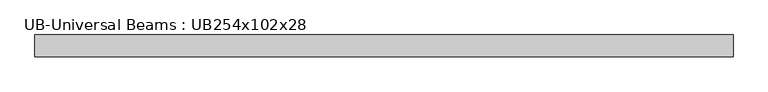
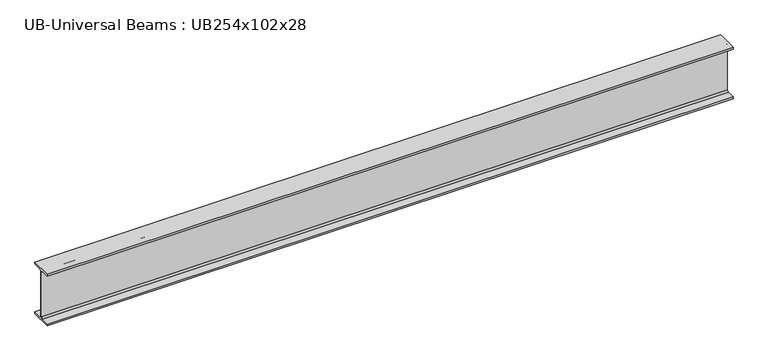
"""IFC4 building model written with IfcOpenShell, lengths in millimetres: beam geometry, UB-Universal Beams : UB254x102x28."""

from ifc_helpers import new_model, si_unit, point, frame, frame_2d, origin, place, context, project, spatial, polyline, circle_curve, trimmed, segment, composite_curve, outline, extrude, source, transform, mapped, element, save


def ub_universal_beams_ub254x102x28_3359efaf(model_context):
    return source(origin(), model_context, "Body", "SweptSolid", [
        extrude(outline(composite_curve([segment(polyline([(51.1, -120.2), (51.1, -130.2), (-51.1, -130.2), (-51.1, -120.2), (-10.75, -120.2)]), True, "CONTINUOUS"), segment(trimmed(circle_curve(frame_2d((-10.75, -112.6)), 7.6), [point((-10.75, -120.2))], [point((-3.15, -112.6))], True, "CARTESIAN"), True, "CONTINUOUS"), segment(polyline([(-3.15, -112.6), (-3.15, 112.6)]), True, "CONTINUOUS"), segment(trimmed(circle_curve(frame_2d((-10.75, 112.6)), 7.6), [point((-3.15, 112.6))], [point((-10.75, 120.2))], True, "CARTESIAN"), True, "CONTINUOUS"), segment(polyline([(-10.75, 120.2), (-51.1, 120.2), (-51.1, 130.2), (51.1, 130.2), (51.1, 120.2), (10.75, 120.2)]), True, "CONTINUOUS"), segment(trimmed(circle_curve(frame_2d((10.75, 112.6)), 7.6), [point((10.75, 120.2))], [point((3.15, 112.6))], True, "CARTESIAN"), True, "CONTINUOUS"), segment(polyline([(3.15, 112.6), (3.15, -112.6)]), True, "CONTINUOUS"), segment(trimmed(circle_curve(frame_2d((10.75, -112.6)), 7.6), [point((3.15, -112.6))], [point((10.75, -120.2))], True, "CARTESIAN"), True, "CONTINUOUS"), segment(polyline([(10.75, -120.2), (51.1, -120.2)]), True, "CONTINUOUS")], self_intersect=False)), frame((-1634.2, 0.0, 0.0), z_axis=(1.0, 0.0, 0.0), x_axis=(0.0, 1.0, 0.0)), (0.0, 0.0, 1.0), 3268.4),
    ])


if __name__ == "__main__":
    model = new_model("IFC4")
    model_context = context("Model", 3, world=origin())
    ifc_project = project(units=[si_unit("LENGTHUNIT", "METRE", prefix="MILLI")], contexts=[model_context])
    site = spatial("IfcSite", under=ifc_project)
    building = spatial("IfcBuilding", under=site)
    placement = place(None, origin())
    ub_universal_beams_ub254x102x28_shape = ub_universal_beams_ub254x102x28_3359efaf(model_context)
    element("IfcBeam", 1, ObjectType="UB-Universal Beams : UB254x102x28", at=placement, inside=building, context=model_context, shape_type="MappedRepresentation", body=[
        mapped(ub_universal_beams_ub254x102x28_shape, transform((0.0, 0.0, 0.0), x_axis=(1.0, 0.0, 0.0), y_axis=(0.0, 1.0, 0.0), z_axis=(0.0, 0.0, 1.0))),
    ])
    save(model, "model.ifc")

# Revit data of these elements
# Type "UB-Universal Beams : UB254x102x28"
#   Section Name Key = "UB254X102X28"
#   Width = 10.22 cm
#   Web Thickness = 0.63 cm
#   Web Fillet = 0.76 cm
#   Warping Constant = 28000.0 cm⁶
#   Torsional Moment of Inertia = 9.57 cm⁴
#   Section Area = 36.1 cm²
#   Plastic Modulus weak axis = 54.8 cm³
#   Plastic Modulus strong axis = 353.0 cm³
#   Nominal Weight = 28.2999 kgf/m
#   Moment of Inertia weak axis = 179.00 cm⁴
#   Moment of Inertia strong axis = 4005.00 cm⁴
#   Height = 26.04 cm
#   Flange Thickness = 1.0 cm
#   Elastic Modulus weak axis = 34.9 cm³
#   Elastic Modulus strong axis = 308.0 cm³
#   Centroid Vertical = 13.02 cm
#   Centroid Horizontal = 5.11 cm
#   Bolt Spacing = 5.4 cm
#   Length [instance default] = 4' - 11.05512"
#   Structural Material [instance default] = Metal - Steel 43-275
#   Type Comments = ""
#   Assembly Code = ""
# Element 1 (IfcBeam, "UB-Universal Beams : UB254x102x28")
#   Materials on its faces: "Metal - Steel 43-275"
# Materials
#   "Metal - Steel 43-275": class "Metal", colour RGB 247 247 247, transparency 0, Cost = 0
